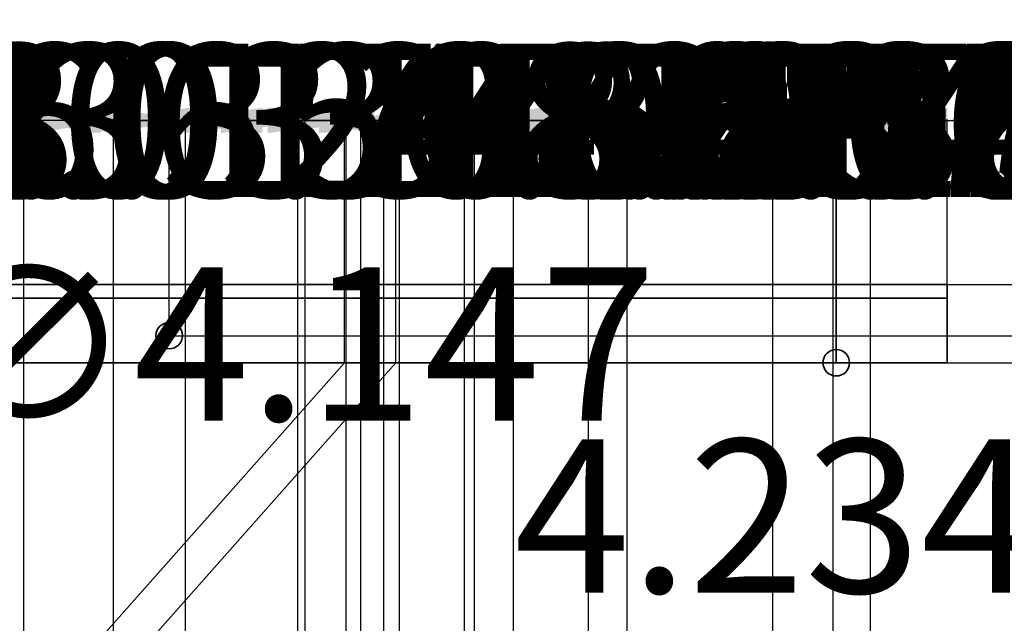
# Model space of a CAD drawing. Units: inches. Extents: x 172 to 828, y 190 to 777.
# Tile 7 of 9: x 474 to 628, y 682 to 777. Entities that reach past the tile are written whole.
import ezdxf

# ---------------------------------------------------------------- set-up
doc = ezdxf.new("R2010")
doc.units = ezdxf.units.IN
doc.header["$MEASUREMENT"] = 0
doc.layers.add('A-ANNO-DIMS', color=2, linetype='Continuous', lineweight=18)
doc.layers.add('A-ELEV', color=7, linetype='Continuous', lineweight=35)
doc.styles.get("Standard").update_dxf_attribs({"font": 'arial.ttf'})
doc.dimstyles.get("Standard").update_dxf_attribs({"dimtxt": 24, "dimasz": 12, "dimexe": 0.18, "dimexo": 0.0625, "dimgap": 0.09, "dimtad": 0, "dimtih": 1, "dimtoh": 1, "dimdec": 0, "dimzin": 0, "dimdsep": 46, "dimlunit": 3, "dimtxsty": 'Standard', "dimcen": 0.09, "dimadec": 0, "dimazin": 0, "dimtfac": 1, "dimtdec": 0, "dimtofl": 0, "dimtmove": 0, "dimatfit": 3, "dimfxl": 1, "dimtolj": 1, "dimtzin": 0, "dimarcsym": 0})

# ---------------------------------------------------------------- blocks, each defined once
blk = doc.blocks.new('*D10')
at = {"layer": 'A-ANNO-DIMS', "color": 0, "lineweight": -2, "transparency": 16777216}
for p, q in [((258.78, 231.45), (258.78, 761.27)), ((270.78, 761.09), (412.23, 761.09)), ((606.78, 761.09), (465.33, 761.09)), ((618.78, 735.45), (618.78, 761.27))]:
    blk.add_line(p, q, dxfattribs=at)
at = {"layer": 'A-ANNO-DIMS', "color": 0, "transparency": 16777216}
for points in [[(270.78, 763.09), (270.78, 759.09), (258.78, 761.09)], [(606.78, 763.09), (606.78, 759.09), (618.78, 761.09)]]:
    blk.add_solid(points, dxfattribs=at)
at = {"layer": 'Defpoints', "color": 0, "transparency": 16777216}
for p in [(618.78, 761.09), (618.78, 735.39), (258.78, 231.39)]:
    blk.add_point(p, dxfattribs=at)
at = {"layer": 'A-ANNO-DIMS', "color": 0, "transparency": 16777216, "insert": (438.78, 761.09), "char_height": 24, "attachment_point": 5}
blk.add_mtext('\\A1;360', dxfattribs=at)
blk = doc.blocks.new('*D11')
at = {"layer": 'A-ANNO-DIMS', "color": 0, "lineweight": -2, "transparency": 16777216}
for p, q in [((618.84, 735.39), (645.16, 735.39)), ((644.98, 723.39), (644.98, 495.74)), ((644.98, 243.39), (644.98, 471.05)), ((618.84, 231.39), (645.16, 231.39))]:
    blk.add_line(p, q, dxfattribs=at)
at = {"layer": 'A-ANNO-DIMS', "color": 0, "transparency": 16777216}
for points in [[(642.98, 723.39), (646.98, 723.39), (644.98, 735.39)], [(642.98, 243.39), (646.98, 243.39), (644.98, 231.39)]]:
    blk.add_solid(points, dxfattribs=at)
at = {"layer": 'Defpoints', "color": 0, "transparency": 16777216}
for p in [(618.78, 735.39), (644.98, 735.39), (618.78, 231.39)]:
    blk.add_point(p, dxfattribs=at)
at = {"layer": 'A-ANNO-DIMS', "color": 0, "transparency": 16777216, "insert": (644.98, 483.39), "char_height": 24, "attachment_point": 5}
blk.add_mtext('\\A1;504', dxfattribs=at)
blk = doc.blocks.new('*D36')
at = {"layer": 'A-ANNO-DIMS', "color": 0, "lineweight": -2, "transparency": 16777216}
for p, q in [((258.78, 735.45), (258.78, 761.27)), ((270.78, 761.09), (412.23, 761.09)), ((606.78, 761.09), (465.33, 761.09)), ((618.78, 735.45), (618.78, 761.27))]:
    blk.add_line(p, q, dxfattribs=at)
at = {"layer": 'A-ANNO-DIMS', "color": 0, "transparency": 16777216}
for points in [[(270.78, 763.09), (270.78, 759.09), (258.78, 761.09)], [(606.78, 763.09), (606.78, 759.09), (618.78, 761.09)]]:
    blk.add_solid(points, dxfattribs=at)
at = {"layer": 'Defpoints', "color": 0, "transparency": 16777216}
for p in [(618.78, 761.09), (258.78, 735.39), (618.78, 735.39)]:
    blk.add_point(p, dxfattribs=at)
at = {"layer": 'A-ANNO-DIMS', "color": 0, "transparency": 16777216, "insert": (438.78, 761.09), "char_height": 24, "attachment_point": 5}
blk.add_mtext('\\A1;360', dxfattribs=at)
blk = doc.blocks.new('*D44')
at = {"layer": 'A-ANNO-DIMS', "color": 0, "lineweight": -2, "transparency": 16777216}
for p, q in [((333.72, 723.23), (333.72, 761.27)), ((345.72, 761.09), (377.1, 761.09)), ((389.1, 727.47), (389.1, 761.27)), ((389.1, 761.09), (401.1, 761.09))]:
    blk.add_line(p, q, dxfattribs=at)
at = {"layer": 'A-ANNO-DIMS', "color": 0, "transparency": 16777216}
for points in [[(345.72, 763.09), (345.72, 759.09), (333.72, 761.09)], [(377.1, 763.09), (377.1, 759.09), (389.1, 761.09)]]:
    blk.add_solid(points, dxfattribs=at)
at = {"layer": 'Defpoints', "color": 0, "transparency": 16777216}
for p in [(389.1, 761.09), (389.1, 727.4), (333.72, 723.17)]:
    blk.add_point(p, dxfattribs=at)
at = {"layer": 'A-ANNO-DIMS', "color": 0, "transparency": 16777216, "insert": (441.71, 761.09), "char_height": 24, "attachment_point": 5}
blk.add_mtext('\\A1;55.38', dxfattribs=at)
blk = doc.blocks.new('*D45')
at = {"layer": 'A-ANNO-DIMS', "color": 0, "lineweight": -2, "transparency": 16777216}
for p, q in [((389.1, 727.47), (389.1, 761.27)), ((401.1, 761.09), (417.14, 761.09)), ((429.14, 615.45), (429.14, 761.27)), ((429.14, 761.09), (441.14, 761.09))]:
    blk.add_line(p, q, dxfattribs=at)
at = {"layer": 'A-ANNO-DIMS', "color": 0, "transparency": 16777216}
for points in [[(401.1, 763.09), (401.1, 759.09), (389.1, 761.09)], [(417.14, 763.09), (417.14, 759.09), (429.14, 761.09)]]:
    blk.add_solid(points, dxfattribs=at)
at = {"layer": 'Defpoints', "color": 0, "transparency": 16777216}
for p in [(429.14, 761.09), (389.1, 727.4), (429.14, 615.39)]:
    blk.add_point(p, dxfattribs=at)
at = {"layer": 'A-ANNO-DIMS', "color": 0, "transparency": 16777216, "insert": (482.2, 761.09), "char_height": 24, "attachment_point": 5}
blk.add_mtext('\\A1;40.03', dxfattribs=at)
blk = doc.blocks.new('*D46')
at = {"layer": 'A-ANNO-DIMS', "color": 0, "lineweight": -2, "transparency": 16777216}
for p, q in [((429.14, 615.45), (429.14, 761.27)), ((441.14, 761.09), (445.77, 761.09)), ((485.14, 761.09), (480.51, 761.09)), ((497.14, 727.47), (497.14, 761.27))]:
    blk.add_line(p, q, dxfattribs=at)
at = {"layer": 'A-ANNO-DIMS', "color": 0, "transparency": 16777216}
for points in [[(441.14, 763.09), (441.14, 759.09), (429.14, 761.09)], [(485.14, 763.09), (485.14, 759.09), (497.14, 761.09)]]:
    blk.add_solid(points, dxfattribs=at)
at = {"layer": 'Defpoints', "color": 0, "transparency": 16777216}
for p in [(497.14, 761.09), (497.14, 727.4), (429.14, 615.39)]:
    blk.add_point(p, dxfattribs=at)
at = {"layer": 'A-ANNO-DIMS', "color": 0, "transparency": 16777216, "insert": (463.14, 761.09), "char_height": 24, "attachment_point": 5}
blk.add_mtext('\\A1;68', dxfattribs=at)
blk = doc.blocks.new('*D47')
at = {"layer": 'A-ANNO-DIMS', "color": 0, "lineweight": -2, "transparency": 16777216}
for p, q in [((497.14, 727.47), (497.14, 761.27)), ((509.14, 761.09), (512.55, 761.09)), ((524.55, 723.23), (524.55, 761.27)), ((524.55, 761.09), (536.55, 761.09))]:
    blk.add_line(p, q, dxfattribs=at)
at = {"layer": 'A-ANNO-DIMS', "color": 0, "transparency": 16777216}
for points in [[(509.14, 763.09), (509.14, 759.09), (497.14, 761.09)], [(512.55, 763.09), (512.55, 759.09), (524.55, 761.09)]]:
    blk.add_solid(points, dxfattribs=at)
at = {"layer": 'Defpoints', "color": 0, "transparency": 16777216}
for p in [(524.55, 761.09), (497.14, 727.4), (524.55, 723.17)]:
    blk.add_point(p, dxfattribs=at)
at = {"layer": 'A-ANNO-DIMS', "color": 0, "transparency": 16777216, "insert": (575.02, 761.09), "char_height": 24, "attachment_point": 5}
blk.add_mtext('\\A1;27.41', dxfattribs=at)
blk = doc.blocks.new('*D48')
at = {"layer": 'A-ANNO-DIMS', "color": 0, "lineweight": -2, "transparency": 16777216}
for p, q in [((512.55, 761.09), (500.55, 761.09)), ((524.55, 723.23), (524.55, 761.27)), ((532.56, 723.23), (532.56, 761.27)), ((544.56, 761.09), (556.56, 761.09))]:
    blk.add_line(p, q, dxfattribs=at)
at = {"layer": 'A-ANNO-DIMS', "color": 0, "transparency": 16777216}
for points in [[(512.55, 763.09), (512.55, 759.09), (524.55, 761.09)], [(544.56, 763.09), (544.56, 759.09), (532.56, 761.09)]]:
    blk.add_solid(points, dxfattribs=at)
at = {"layer": 'Defpoints', "color": 0, "transparency": 16777216}
for p in [(532.56, 761.09), (524.55, 723.17), (532.56, 723.17)]:
    blk.add_point(p, dxfattribs=at)
at = {"layer": 'A-ANNO-DIMS', "color": 0, "transparency": 16777216, "insert": (597.16, 761.09), "char_height": 24, "attachment_point": 5}
blk.add_mtext('\\A1;8.013', dxfattribs=at)
blk = doc.blocks.new('*D49')
at = {"layer": 'A-ANNO-DIMS', "color": 0, "lineweight": -2, "transparency": 16777216}
for p, q in [((520.563677, 761.092291), (508.563677, 761.092291)), ((532.563677, 723.230871), (532.563677, 761.272291)), ((601.465061, 723.230871), (601.465061, 761.272291)), ((613.465061, 761.092291), (625.465061, 761.092291))]:
    blk.add_line(p, q, dxfattribs=at)
at = {"layer": 'A-ANNO-DIMS', "color": 0, "transparency": 16777216}
for points in [[(520.563677, 763.092291), (520.563677, 759.092291), (532.563677, 761.092291)], [(613.465061, 763.092291), (613.465061, 759.092291), (601.465061, 761.092291)]]:
    blk.add_solid(points, dxfattribs=at)
at = {"layer": 'Defpoints', "color": 0, "transparency": 16777216}
for p in [(601.465061, 761.092291), (532.563677, 723.168371), (601.465061, 723.168371)]:
    blk.add_point(p, dxfattribs=at)
at = {"layer": 'A-ANNO-DIMS', "color": 0, "transparency": 16777216, "insert": (567.014369, 761.092291), "char_height": 24, "attachment_point": 5}
blk.add_mtext('\\A1;68.9', dxfattribs=at)
blk = doc.blocks.new('*D50')
at = {"layer": 'A-ANNO-DIMS', "color": 0, "lineweight": -2, "transparency": 16777216}
for p, q in [((589.47, 761.09), (577.47, 761.09)), ((601.47, 723.23), (601.47, 761.27)), ((618.78, 735.45), (618.78, 761.27)), ((630.78, 761.09), (642.78, 761.09))]:
    blk.add_line(p, q, dxfattribs=at)
at = {"layer": 'A-ANNO-DIMS', "color": 0, "transparency": 16777216}
for points in [[(589.47, 763.09), (589.47, 759.09), (601.47, 761.09)], [(630.78, 763.09), (630.78, 759.09), (618.78, 761.09)]]:
    blk.add_solid(points, dxfattribs=at)
at = {"layer": 'Defpoints', "color": 0, "transparency": 16777216}
for p in [(618.78, 761.09), (618.78, 735.39), (601.47, 723.17)]:
    blk.add_point(p, dxfattribs=at)
at = {"layer": 'A-ANNO-DIMS', "color": 0, "transparency": 16777216, "insert": (691.51, 761.09), "char_height": 24, "attachment_point": 5}
blk.add_mtext('\\A1;17.314', dxfattribs=at)
blk = doc.blocks.new('*D51')
at = {"layer": 'A-ANNO-DIMS', "color": 0, "lineweight": -2, "transparency": 16777216}
for p, q in [((644.98, 739.4), (644.98, 751.4)), ((497.2, 727.4), (645.16, 727.4)), ((601.53, 723.17), (645.16, 723.17)), ((644.98, 711.17), (644.98, 699.17)), ((644.98, 699.17), (632.98, 699.17))]:
    blk.add_line(p, q, dxfattribs=at)
at = {"layer": 'A-ANNO-DIMS', "color": 0, "transparency": 16777216}
for points in [[(642.98, 739.4), (646.98, 739.4), (644.98, 727.4)], [(642.98, 711.17), (646.98, 711.17), (644.98, 723.17)]]:
    blk.add_solid(points, dxfattribs=at)
at = {"layer": 'Defpoints', "color": 0, "transparency": 16777216}
for p in [(497.14, 727.4), (601.47, 723.17), (644.98, 723.17)]:
    blk.add_point(p, dxfattribs=at)
at = {"layer": 'A-ANNO-DIMS', "color": 0, "transparency": 16777216, "insert": (591.96, 699.17), "char_height": 24, "attachment_point": 5}
blk.add_mtext('\\A1;4.234', dxfattribs=at)
blk = doc.blocks.new('*D52')
at = {"layer": 'A-ANNO-DIMS', "color": 0, "lineweight": -2, "transparency": 16777216}
for p, q in [((409.12, 761.09), (397.12, 761.09)), ((421.12, 615.45), (421.12, 761.27)), ((429.14, 615.45), (429.14, 761.27)), ((441.14, 761.09), (453.14, 761.09))]:
    blk.add_line(p, q, dxfattribs=at)
at = {"layer": 'A-ANNO-DIMS', "color": 0, "transparency": 16777216}
for points in [[(409.12, 763.09), (409.12, 759.09), (421.12, 761.09)], [(441.14, 763.09), (441.14, 759.09), (429.14, 761.09)]]:
    blk.add_solid(points, dxfattribs=at)
at = {"layer": 'Defpoints', "color": 0, "transparency": 16777216}
for p in [(429.14, 761.09), (421.12, 615.39), (429.14, 615.39)]:
    blk.add_point(p, dxfattribs=at)
at = {"layer": 'A-ANNO-DIMS', "color": 0, "transparency": 16777216, "insert": (493.74, 761.09), "char_height": 24, "attachment_point": 5}
blk.add_mtext('\\A1;8.013', dxfattribs=at)
blk = doc.blocks.new('*D53')
at = {"layer": 'A-ANNO-DIMS', "color": 0, "lineweight": -2, "transparency": 16777216}
for p, q in [((417.14, 761.09), (405.14, 761.09)), ((429.14, 615.45), (429.14, 761.27)), ((437.15, 615.45), (437.15, 761.27)), ((449.15, 761.09), (461.15, 761.09))]:
    blk.add_line(p, q, dxfattribs=at)
at = {"layer": 'A-ANNO-DIMS', "color": 0, "transparency": 16777216}
for points in [[(417.14, 763.09), (417.14, 759.09), (429.14, 761.09)], [(449.15, 763.09), (449.15, 759.09), (437.15, 761.09)]]:
    blk.add_solid(points, dxfattribs=at)
at = {"layer": 'Defpoints', "color": 0, "transparency": 16777216}
for p in [(437.15, 761.09), (429.14, 615.39), (437.15, 615.39)]:
    blk.add_point(p, dxfattribs=at)
at = {"layer": 'A-ANNO-DIMS', "color": 0, "transparency": 16777216, "insert": (501.75, 761.09), "char_height": 24, "attachment_point": 5}
blk.add_mtext('\\A1;8.013', dxfattribs=at)
blk = doc.blocks.new('*D54')
at = {"layer": 'A-ANNO-DIMS', "color": 0, "lineweight": -2, "transparency": 16777216}
for p, q in [((267.48, 615.45), (267.48, 761.27)), ((279.48, 761.09), (330.13, 761.09)), ((462.39, 761.09), (411.75, 761.09)), ((474.39, 633.61), (474.39, 761.27))]:
    blk.add_line(p, q, dxfattribs=at)
at = {"layer": 'A-ANNO-DIMS', "color": 0, "transparency": 16777216}
for points in [[(279.48, 763.09), (279.48, 759.09), (267.48, 761.09)], [(462.39, 763.09), (462.39, 759.09), (474.39, 761.09)]]:
    blk.add_solid(points, dxfattribs=at)
at = {"layer": 'Defpoints', "color": 0, "transparency": 16777216}
for p in [(474.39, 761.09), (474.39, 633.55), (267.48, 615.39)]:
    blk.add_point(p, dxfattribs=at)
at = {"layer": 'A-ANNO-DIMS', "color": 0, "transparency": 16777216, "insert": (370.94, 761.09), "char_height": 24, "attachment_point": 5}
blk.add_mtext('\\A1;206.9', dxfattribs=at)
blk = doc.blocks.new('*D55')
at = {"layer": 'A-ANNO-DIMS', "color": 0, "lineweight": -2, "transparency": 16777216}
for p, q in [((474.39, 633.61), (474.39, 761.27)), ((486.39, 761.09), (506.4, 761.09)), ((518.4, 633.61), (518.4, 761.27)), ((518.4, 761.09), (530.4, 761.09))]:
    blk.add_line(p, q, dxfattribs=at)
at = {"layer": 'A-ANNO-DIMS', "color": 0, "transparency": 16777216}
for points in [[(486.39, 763.09), (486.39, 759.09), (474.39, 761.09)], [(506.4, 763.09), (506.4, 759.09), (518.4, 761.09)]]:
    blk.add_solid(points, dxfattribs=at)
at = {"layer": 'Defpoints', "color": 0, "transparency": 16777216}
for p in [(518.4, 761.09), (474.39, 633.55), (518.4, 633.55)]:
    blk.add_point(p, dxfattribs=at)
at = {"layer": 'A-ANNO-DIMS', "color": 0, "transparency": 16777216, "insert": (569.15, 761.09), "char_height": 24, "attachment_point": 5}
blk.add_mtext('\\A1;44.01', dxfattribs=at)
blk = doc.blocks.new('*D56')
at = {"layer": 'A-ANNO-DIMS', "color": 0, "lineweight": -2, "transparency": 16777216}
for p, q in [((506.4, 761.09), (494.4, 761.09)), ((518.4, 633.61), (518.4, 761.27)), ((527.09, 657.43), (527.09, 761.27)), ((539.09, 761.09), (551.09, 761.09))]:
    blk.add_line(p, q, dxfattribs=at)
at = {"layer": 'A-ANNO-DIMS', "color": 0, "transparency": 16777216}
for points in [[(506.4, 763.09), (506.4, 759.09), (518.4, 761.09)], [(539.09, 763.09), (539.09, 759.09), (527.09, 761.09)]]:
    blk.add_solid(points, dxfattribs=at)
at = {"layer": 'Defpoints', "color": 0, "transparency": 16777216}
for p in [(527.09, 761.09), (527.09, 657.37), (518.4, 633.55)]:
    blk.add_point(p, dxfattribs=at)
at = {"layer": 'A-ANNO-DIMS', "color": 0, "transparency": 16777216, "insert": (582.4, 761.09), "char_height": 24, "attachment_point": 5}
blk.add_mtext('\\A1;8.69', dxfattribs=at)
blk = doc.blocks.new('*D57')
at = {"layer": 'A-ANNO-DIMS', "color": 0, "lineweight": -2, "transparency": 16777216}
for p, q in [((515.09, 761.09), (503.09, 761.09)), ((527.09, 657.43), (527.09, 761.27)), ((533.17, 657.43), (533.17, 761.27)), ((545.17, 761.09), (557.17, 761.09))]:
    blk.add_line(p, q, dxfattribs=at)
at = {"layer": 'A-ANNO-DIMS', "color": 0, "transparency": 16777216}
for points in [[(515.09, 763.09), (515.09, 759.09), (527.09, 761.09)], [(545.17, 763.09), (545.17, 759.09), (533.17, 761.09)]]:
    blk.add_solid(points, dxfattribs=at)
at = {"layer": 'Defpoints', "color": 0, "transparency": 16777216}
for p in [(533.17, 761.09), (527.09, 657.37), (533.17, 657.37)]:
    blk.add_point(p, dxfattribs=at)
at = {"layer": 'A-ANNO-DIMS', "color": 0, "transparency": 16777216, "insert": (597.85, 761.09), "char_height": 24, "attachment_point": 5}
blk.add_mtext('\\A1;6.078', dxfattribs=at)
blk = doc.blocks.new('*D58')
at = {"layer": 'A-ANNO-DIMS', "color": 0, "lineweight": -2, "transparency": 16777216}
for p, q in [((521.17, 761.09), (509.17, 761.09)), ((533.17, 657.43), (533.17, 761.27)), ((544.89, 657.43), (544.89, 761.27)), ((556.89, 761.09), (568.89, 761.09))]:
    blk.add_line(p, q, dxfattribs=at)
at = {"layer": 'A-ANNO-DIMS', "color": 0, "transparency": 16777216}
for points in [[(521.17, 763.09), (521.17, 759.09), (533.17, 761.09)], [(556.89, 763.09), (556.89, 759.09), (544.89, 761.09)]]:
    blk.add_solid(points, dxfattribs=at)
at = {"layer": 'Defpoints', "color": 0, "transparency": 16777216}
for p in [(544.89, 761.09), (533.17, 657.37), (544.89, 657.37)]:
    blk.add_point(p, dxfattribs=at)
at = {"layer": 'A-ANNO-DIMS', "color": 0, "transparency": 16777216, "insert": (608.22, 761.09), "char_height": 24, "attachment_point": 5}
blk.add_mtext('\\A1;11.72', dxfattribs=at)
blk = doc.blocks.new('*D59')
at = {"layer": 'A-ANNO-DIMS', "color": 0, "lineweight": -2, "transparency": 16777216}
for p, q in [((532.89, 761.09), (520.89, 761.09)), ((544.89, 657.43), (544.89, 761.27)), ((550.97, 657.43), (550.97, 761.27)), ((562.97, 761.09), (574.97, 761.09))]:
    blk.add_line(p, q, dxfattribs=at)
at = {"layer": 'A-ANNO-DIMS', "color": 0, "transparency": 16777216}
for points in [[(532.89, 763.09), (532.89, 759.09), (544.89, 761.09)], [(562.97, 763.09), (562.97, 759.09), (550.97, 761.09)]]:
    blk.add_solid(points, dxfattribs=at)
at = {"layer": 'Defpoints', "color": 0, "transparency": 16777216}
for p in [(550.97, 761.09), (544.89, 657.37), (550.97, 657.37)]:
    blk.add_point(p, dxfattribs=at)
at = {"layer": 'A-ANNO-DIMS', "color": 0, "transparency": 16777216, "insert": (615.64, 761.09), "char_height": 24, "attachment_point": 5}
blk.add_mtext('\\A1;6.078', dxfattribs=at)
blk = doc.blocks.new('*D60')
at = {"layer": 'A-ANNO-DIMS', "color": 0, "lineweight": -2, "transparency": 16777216}
for p, q in [((538.97, 761.09), (526.97, 761.09)), ((550.97, 657.43), (550.97, 761.27)), ((562.69, 657.43), (562.69, 761.27)), ((574.69, 761.09), (586.69, 761.09))]:
    blk.add_line(p, q, dxfattribs=at)
at = {"layer": 'A-ANNO-DIMS', "color": 0, "transparency": 16777216}
for points in [[(538.97, 763.09), (538.97, 759.09), (550.97, 761.09)], [(574.69, 763.09), (574.69, 759.09), (562.69, 761.09)]]:
    blk.add_solid(points, dxfattribs=at)
at = {"layer": 'Defpoints', "color": 0, "transparency": 16777216}
for p in [(562.69, 761.09), (550.97, 657.37), (562.69, 657.37)]:
    blk.add_point(p, dxfattribs=at)
at = {"layer": 'A-ANNO-DIMS', "color": 0, "transparency": 16777216, "insert": (626.02, 761.09), "char_height": 24, "attachment_point": 5}
blk.add_mtext('\\A1;11.72', dxfattribs=at)
blk = doc.blocks.new('*D61')
at = {"layer": 'A-ANNO-DIMS', "color": 0, "lineweight": -2, "transparency": 16777216}
for p, q in [((550.69, 761.09), (538.69, 761.09)), ((562.69, 657.43), (562.69, 761.27)), ((568.77, 657.43), (568.77, 761.27)), ((580.77, 761.09), (592.77, 761.09))]:
    blk.add_line(p, q, dxfattribs=at)
at = {"layer": 'A-ANNO-DIMS', "color": 0, "transparency": 16777216}
for points in [[(550.69, 763.09), (550.69, 759.09), (562.69, 761.09)], [(580.77, 763.09), (580.77, 759.09), (568.77, 761.09)]]:
    blk.add_solid(points, dxfattribs=at)
at = {"layer": 'Defpoints', "color": 0, "transparency": 16777216}
for p in [(568.77, 761.09), (562.69, 657.37), (568.77, 657.37)]:
    blk.add_point(p, dxfattribs=at)
at = {"layer": 'A-ANNO-DIMS', "color": 0, "transparency": 16777216, "insert": (633.44, 761.09), "char_height": 24, "attachment_point": 5}
blk.add_mtext('\\A1;6.078', dxfattribs=at)
blk = doc.blocks.new('*D62')
at = {"layer": 'A-ANNO-DIMS', "color": 0, "lineweight": -2, "transparency": 16777216}
for p, q in [((568.77, 657.43), (568.77, 761.27)), ((580.77, 761.09), (594.82, 761.09)), ((606.82, 663.45), (606.82, 761.27)), ((606.82, 761.09), (618.82, 761.09))]:
    blk.add_line(p, q, dxfattribs=at)
at = {"layer": 'A-ANNO-DIMS', "color": 0, "transparency": 16777216}
for points in [[(580.77, 763.09), (580.77, 759.09), (568.77, 761.09)], [(594.82, 763.09), (594.82, 759.09), (606.82, 761.09)]]:
    blk.add_solid(points, dxfattribs=at)
at = {"layer": 'Defpoints', "color": 0, "transparency": 16777216}
for p in [(606.82, 761.09), (606.82, 663.39), (568.77, 657.37)]:
    blk.add_point(p, dxfattribs=at)
at = {"layer": 'A-ANNO-DIMS', "color": 0, "transparency": 16777216, "insert": (659.48, 761.09), "char_height": 24, "attachment_point": 5}
blk.add_mtext('\\A1;38.05', dxfattribs=at)
blk = doc.blocks.new('*D63')
at = {"layer": 'A-ANNO-DIMS', "color": 0, "lineweight": -2, "transparency": 16777216}
for p, q in [((594.82, 761.09), (582.82, 761.09)), ((606.82, 663.45), (606.82, 761.27)), ((618.78, 723.23), (618.78, 761.27)), ((630.78, 761.09), (642.78, 761.09))]:
    blk.add_line(p, q, dxfattribs=at)
at = {"layer": 'A-ANNO-DIMS', "color": 0, "transparency": 16777216}
for points in [[(594.82, 763.09), (594.82, 759.09), (606.82, 761.09)], [(630.78, 763.09), (630.78, 759.09), (618.78, 761.09)]]:
    blk.add_solid(points, dxfattribs=at)
at = {"layer": 'Defpoints', "color": 0, "transparency": 16777216}
for p in [(618.78, 761.09), (618.78, 723.17), (606.82, 663.39)]:
    blk.add_point(p, dxfattribs=at)
at = {"layer": 'A-ANNO-DIMS', "color": 0, "transparency": 16777216, "insert": (691.56, 761.09), "char_height": 24, "attachment_point": 5}
blk.add_mtext('\\A1;11.963', dxfattribs=at)
blk = doc.blocks.new('*D76')
at = {"layer": 'A-ANNO-DIMS', "color": 0, "lineweight": -2, "transparency": 16777216}
for p, q in [((399.24, 761.09), (387.24, 761.09)), ((411.24, 495.45), (411.24, 761.27)), ((427.59, 495.45), (427.59, 761.27)), ((439.59, 761.09), (451.59, 761.09))]:
    blk.add_line(p, q, dxfattribs=at)
at = {"layer": 'A-ANNO-DIMS', "color": 0, "transparency": 16777216}
for points in [[(399.24, 763.09), (399.24, 759.09), (411.24, 761.09)], [(439.59, 763.09), (439.59, 759.09), (427.59, 761.09)]]:
    blk.add_solid(points, dxfattribs=at)
at = {"layer": 'Defpoints', "color": 0, "transparency": 16777216}
for p in [(427.59, 761.09), (411.24, 495.39), (427.59, 495.39)]:
    blk.add_point(p, dxfattribs=at)
at = {"layer": 'A-ANNO-DIMS', "color": 0, "transparency": 16777216, "insert": (500.36, 761.09), "char_height": 24, "attachment_point": 5}
blk.add_mtext('\\A1;16.356', dxfattribs=at)
blk = doc.blocks.new('*D77')
at = {"layer": 'A-ANNO-DIMS', "color": 0, "lineweight": -2, "transparency": 16777216}
for p, q in [((427.59, 495.45), (427.59, 761.27)), ((439.59, 761.09), (452.34, 761.09)), ((464.34, 495.45), (464.34, 761.27)), ((464.34, 761.09), (476.34, 761.09))]:
    blk.add_line(p, q, dxfattribs=at)
at = {"layer": 'A-ANNO-DIMS', "color": 0, "transparency": 16777216}
for points in [[(439.59, 763.09), (439.59, 759.09), (427.59, 761.09)], [(452.34, 763.09), (452.34, 759.09), (464.34, 761.09)]]:
    blk.add_solid(points, dxfattribs=at)
at = {"layer": 'Defpoints', "color": 0, "transparency": 16777216}
for p in [(464.34, 761.09), (427.59, 495.39), (464.34, 495.39)]:
    blk.add_point(p, dxfattribs=at)
at = {"layer": 'A-ANNO-DIMS', "color": 0, "transparency": 16777216, "insert": (516.86, 761.09), "char_height": 24, "attachment_point": 5}
blk.add_mtext('\\A1;36.74', dxfattribs=at)
blk = doc.blocks.new('*D78')
at = {"layer": 'A-ANNO-DIMS', "color": 0, "lineweight": -2, "transparency": 16777216}
for p, q in [((452.34, 761.09), (440.34, 761.09)), ((464.34, 607.45), (464.34, 761.27)), ((488.42, 607.45), (488.42, 761.27)), ((500.42, 761.09), (512.42, 761.09))]:
    blk.add_line(p, q, dxfattribs=at)
at = {"layer": 'A-ANNO-DIMS', "color": 0, "transparency": 16777216}
for points in [[(452.34, 763.09), (452.34, 759.09), (464.34, 761.09)], [(500.42, 763.09), (500.42, 759.09), (488.42, 761.09)]]:
    blk.add_solid(points, dxfattribs=at)
at = {"layer": 'Defpoints', "color": 0, "transparency": 16777216}
for p in [(488.42, 761.09), (464.34, 607.39), (488.42, 607.39)]:
    blk.add_point(p, dxfattribs=at)
at = {"layer": 'A-ANNO-DIMS', "color": 0, "transparency": 16777216, "insert": (562.56, 761.09), "char_height": 24, "attachment_point": 5}
blk.add_mtext('\\A1;24.088', dxfattribs=at)
blk = doc.blocks.new('*D79')
at = {"layer": 'A-ANNO-DIMS', "color": 0, "lineweight": -2, "transparency": 16777216}
for p, q in [((476.42, 761.09), (464.42, 761.09)), ((488.42, 607.45), (488.42, 761.27)), ((499.69, 607.45), (499.69, 761.27)), ((511.69, 761.09), (523.69, 761.09))]:
    blk.add_line(p, q, dxfattribs=at)
at = {"layer": 'A-ANNO-DIMS', "color": 0, "transparency": 16777216}
for points in [[(476.42, 763.09), (476.42, 759.09), (488.42, 761.09)], [(511.69, 763.09), (511.69, 759.09), (499.69, 761.09)]]:
    blk.add_solid(points, dxfattribs=at)
at = {"layer": 'Defpoints', "color": 0, "transparency": 16777216}
for p in [(499.69, 761.09), (488.42, 607.39), (499.69, 607.39)]:
    blk.add_point(p, dxfattribs=at)
at = {"layer": 'A-ANNO-DIMS', "color": 0, "transparency": 16777216, "insert": (563.15, 761.09), "char_height": 24, "attachment_point": 5}
blk.add_mtext('\\A1;11.27', dxfattribs=at)
blk = doc.blocks.new('*D80')
at = {"layer": 'A-ANNO-DIMS', "color": 0, "lineweight": -2, "transparency": 16777216}
for p, q in [((487.69, 761.09), (475.69, 761.09)), ((499.69, 607.45), (499.69, 761.27)), ((517.23, 607.45), (517.23, 761.27)), ((529.23, 761.09), (541.23, 761.09))]:
    blk.add_line(p, q, dxfattribs=at)
at = {"layer": 'A-ANNO-DIMS', "color": 0, "transparency": 16777216}
for points in [[(487.69, 763.09), (487.69, 759.09), (499.69, 761.09)], [(529.23, 763.09), (529.23, 759.09), (517.23, 761.09)]]:
    blk.add_solid(points, dxfattribs=at)
at = {"layer": 'Defpoints', "color": 0, "transparency": 16777216}
for p in [(517.23, 761.09), (499.69, 607.39), (517.23, 607.39)]:
    blk.add_point(p, dxfattribs=at)
at = {"layer": 'A-ANNO-DIMS', "color": 0, "transparency": 16777216, "insert": (590, 761.09), "char_height": 24, "attachment_point": 5}
blk.add_mtext('\\A1;17.533', dxfattribs=at)
blk = doc.blocks.new('*D81')
at = {"layer": 'A-ANNO-DIMS', "color": 0, "lineweight": -2, "transparency": 16777216}
for p, q in [((505.23, 761.09), (493.23, 761.09)), ((517.23, 607.45), (517.23, 761.27)), ((524.83, 493.45), (524.83, 761.27)), ((536.83, 761.09), (548.83, 761.09))]:
    blk.add_line(p, q, dxfattribs=at)
at = {"layer": 'A-ANNO-DIMS', "color": 0, "transparency": 16777216}
for points in [[(505.23, 763.09), (505.23, 759.09), (517.23, 761.09)], [(536.83, 763.09), (536.83, 759.09), (524.83, 761.09)]]:
    blk.add_solid(points, dxfattribs=at)
at = {"layer": 'Defpoints', "color": 0, "transparency": 16777216}
for p in [(524.83, 761.09), (517.23, 607.39), (524.83, 493.39)]:
    blk.add_point(p, dxfattribs=at)
at = {"layer": 'A-ANNO-DIMS', "color": 0, "transparency": 16777216, "insert": (570.66, 761.09), "char_height": 24, "attachment_point": 5}
blk.add_mtext('\\A1;7.6', dxfattribs=at)
blk = doc.blocks.new('*D82')
at = {"layer": 'A-ANNO-DIMS', "color": 0, "lineweight": -2, "transparency": 16777216}
for p, q in [((588.96, 761.09), (576.96, 761.09)), ((600.96, 493.45), (600.96, 761.27)), ((606.82, 607.45), (606.82, 761.27)), ((618.82, 761.09), (630.82, 761.09))]:
    blk.add_line(p, q, dxfattribs=at)
at = {"layer": 'A-ANNO-DIMS', "color": 0, "transparency": 16777216}
for points in [[(588.96, 763.09), (588.96, 759.09), (600.96, 761.09)], [(618.82, 763.09), (618.82, 759.09), (606.82, 761.09)]]:
    blk.add_solid(points, dxfattribs=at)
at = {"layer": 'Defpoints', "color": 0, "transparency": 16777216}
for p in [(606.82, 761.09), (606.82, 607.39), (600.96, 493.39)]:
    blk.add_point(p, dxfattribs=at)
at = {"layer": 'A-ANNO-DIMS', "color": 0, "transparency": 16777216, "insert": (671.39, 761.09), "char_height": 24, "attachment_point": 5}
blk.add_mtext('\\A1;5.856', dxfattribs=at)
blk = doc.blocks.new('*D83')
at = {"layer": 'A-ANNO-DIMS', "color": 0, "lineweight": -2, "transparency": 16777216}
for p, q in [((512.83, 761.09), (500.83, 761.09)), ((524.83, 535.45), (524.83, 761.27)), ((543.3, 599.86), (543.3, 761.27)), ((555.3, 761.09), (567.3, 761.09))]:
    blk.add_line(p, q, dxfattribs=at)
at = {"layer": 'A-ANNO-DIMS', "color": 0, "transparency": 16777216}
for points in [[(512.83, 763.09), (512.83, 759.09), (524.83, 761.09)], [(555.3, 763.09), (555.3, 759.09), (543.3, 761.09)]]:
    blk.add_solid(points, dxfattribs=at)
at = {"layer": 'Defpoints', "color": 0, "transparency": 16777216}
for p in [(543.3, 761.09), (543.3, 599.8), (524.83, 535.39)]:
    blk.add_point(p, dxfattribs=at)
at = {"layer": 'A-ANNO-DIMS', "color": 0, "transparency": 16777216, "insert": (606.75, 761.09), "char_height": 24, "attachment_point": 5}
blk.add_mtext('\\A1;18.47', dxfattribs=at)
blk = doc.blocks.new('*D84')
at = {"layer": 'A-ANNO-DIMS', "color": 0, "lineweight": -2, "transparency": 16777216}
for p, q in [((543.3, 599.86), (543.3, 761.27)), ((555.3, 761.09), (579.54, 761.09)), ((591.54, 599.86), (591.54, 761.27)), ((591.54, 761.09), (603.54, 761.09))]:
    blk.add_line(p, q, dxfattribs=at)
at = {"layer": 'A-ANNO-DIMS', "color": 0, "transparency": 16777216}
for points in [[(555.3, 763.09), (555.3, 759.09), (543.3, 761.09)], [(579.54, 763.09), (579.54, 759.09), (591.54, 761.09)]]:
    blk.add_solid(points, dxfattribs=at)
at = {"layer": 'Defpoints', "color": 0, "transparency": 16777216}
for p in [(591.54, 761.09), (543.3, 599.8), (591.54, 599.8)]:
    blk.add_point(p, dxfattribs=at)
at = {"layer": 'A-ANNO-DIMS', "color": 0, "transparency": 16777216, "insert": (644.7, 761.09), "char_height": 24, "attachment_point": 5}
blk.add_mtext('\\A1;48.25', dxfattribs=at)
blk = doc.blocks.new('*D85')
at = {"layer": 'A-ANNO-DIMS', "color": 0, "lineweight": -2, "transparency": 16777216}
for p, q in [((579.54, 761.09), (567.54, 761.09)), ((591.54, 599.86), (591.54, 761.27)), ((600.96, 535.45), (600.96, 761.27)), ((612.96, 761.09), (624.96, 761.09))]:
    blk.add_line(p, q, dxfattribs=at)
at = {"layer": 'A-ANNO-DIMS', "color": 0, "transparency": 16777216}
for points in [[(579.54, 763.09), (579.54, 759.09), (591.54, 761.09)], [(612.96, 763.09), (612.96, 759.09), (600.96, 761.09)]]:
    blk.add_solid(points, dxfattribs=at)
at = {"layer": 'Defpoints', "color": 0, "transparency": 16777216}
for p in [(600.96, 761.09), (591.54, 599.8), (600.96, 535.39)]:
    blk.add_point(p, dxfattribs=at)
at = {"layer": 'A-ANNO-DIMS', "color": 0, "transparency": 16777216, "insert": (665.63, 761.09), "char_height": 24, "attachment_point": 5}
blk.add_mtext('\\A1;9.415', dxfattribs=at)
blk = doc.blocks.new('*D86')
at = {"layer": 'A-ANNO-DIMS', "color": 0, "lineweight": -2, "transparency": 16777216}
for p, q in [((512.83, 761.09), (500.83, 761.09)), ((524.83, 493.45), (524.83, 761.27)), ((530.68, 493.45), (530.68, 761.27)), ((542.68, 761.09), (554.68, 761.09))]:
    blk.add_line(p, q, dxfattribs=at)
at = {"layer": 'A-ANNO-DIMS', "color": 0, "transparency": 16777216}
for points in [[(512.83, 763.09), (512.83, 759.09), (524.83, 761.09)], [(542.68, 763.09), (542.68, 759.09), (530.68, 761.09)]]:
    blk.add_solid(points, dxfattribs=at)
at = {"layer": 'Defpoints', "color": 0, "transparency": 16777216}
for p in [(530.68, 761.09), (524.83, 493.39), (530.68, 493.39)]:
    blk.add_point(p, dxfattribs=at)
at = {"layer": 'A-ANNO-DIMS', "color": 0, "transparency": 16777216, "insert": (595.26, 761.09), "char_height": 24, "attachment_point": 5}
blk.add_mtext('\\A1;5.856', dxfattribs=at)
blk = doc.blocks.new('*D92')
at = {"layer": 'A-ANNO-DIMS', "color": 0, "lineweight": -2, "transparency": 16777216}
for p, q in [((389.01, 727.4), (389.19, 727.4)), ((389.1, 727.31), (389.1, 727.49)), ((415.15, 726.11), (403.16, 726.7))]:
    blk.add_line(p, q, dxfattribs=at)
at = {"layer": 'A-ANNO-DIMS', "color": 0, "transparency": 16777216}
blk.add_solid([(403.26, 728.7), (403.06, 724.71), (391.17, 727.3)], dxfattribs=at)
at = {"layer": 'Defpoints', "color": 0, "transparency": 16777216}
for p in [(387.03, 727.51), (391.17, 727.3)]:
    blk.add_point(p, dxfattribs=at)
at = {"layer": 'A-ANNO-DIMS', "color": 0, "transparency": 16777216, "insert": (493.92, 726.11), "char_height": 24, "attachment_point": 5}
blk.add_mtext('\\A1;3X ∅4.147', dxfattribs=at)

msp = doc.modelspace()

# ---------------------------------------------------------------- linework, layer by layer
at = {"layer": 'A-ELEV'}
for p, q in [((618.7792, 735.3923), (267.4822, 735.3923)), ((618.7792, 735.3923), (618.7792, 733.2598)), ((618.7792, 733.2598), (258.7792, 733.2598)), ((618.7792, 733.2598), (618.7792, 723.1684)), ((618.7792, 723.1684), (258.7792, 723.1684)), ((429.1355, 615.3923), (524.5502, 723.1684)), ((437.149, 615.3923), (532.5637, 723.1684))]:
    msp.add_line(p, q, dxfattribs=at)
for centre in [(497.1421, 727.4027), (601.4651, 723.1684)]:
    msp.add_circle(centre, 2.0735, dxfattribs=at)

# ---------------------------------------------------------------- dimensions: what is measured, and where the dimension line sits
at = {"layer": 'A-ANNO-DIMS'}
for base, p1, p2, override, picture, middle in [((618.7792, 761.0923), (258.7792, 231.3923), (618.7792, 735.3923), {"dimdec": 0, "dimlfac": 1, "dimrnd": 0, "dimzin": 0, "dimdsep": 46, "dimlunit": 2}, '*D10', (438.7792, 761.0923)), ((618.7792, 761.0923), (258.7792, 735.3923), (618.7792, 735.3923), {"dimdec": 0, "dimlfac": 1, "dimrnd": 0, "dimzin": 0, "dimdsep": 46, "dimlunit": 2}, '*D36', (438.7792, 761.0923)), ((474.3939, 761.0923), (267.4822, 615.3923), (474.3939, 633.5521), {"dimdec": 1, "dimlfac": 1, "dimrnd": 0, "dimzin": 0, "dimdsep": 46, "dimlunit": 2}, '*D54', (370.9381, 761.0923)), ((389.104, 761.0923), (333.7209, 723.1684), (389.104, 727.4027), {"dimdec": 2, "dimlfac": 1, "dimrnd": 0, "dimzin": 0, "dimdsep": 46, "dimlunit": 2}, '*D44', (441.7124, 761.0923)), ((427.5926, 761.0923), (411.2362, 495.3923), (427.5926, 495.3923), {"dimdec": 3, "dimlfac": 1, "dimrnd": 0, "dimzin": 0, "dimdsep": 46, "dimlunit": 2}, '*D76', (500.362, 761.0923)), ((429.1355, 761.0923), (389.104, 727.4027), (429.1355, 615.3923), {"dimdec": 2, "dimlfac": 1, "dimrnd": 0, "dimzin": 0, "dimdsep": 46, "dimlunit": 2}, '*D45', (482.2024, 761.0923)), ((429.1355, 761.0923), (421.1221, 615.3923), (429.1355, 615.3923), {"dimdec": 3, "dimlfac": 1, "dimrnd": 0, "dimzin": 0, "dimdsep": 46, "dimlunit": 2}, '*D52', (493.7358, 761.0923)), ((437.149, 761.09229), (429.13555, 615.39229), (437.149, 615.39229), {"dimdec": 3, "dimlfac": 1, "dimrnd": 0, "dimzin": 0, "dimdsep": 46, "dimlunit": 2}, '*D53', (501.74924, 761.09229)), ((464.3356, 761.0923), (427.5926, 495.3923), (464.3356, 495.3923), {"dimdec": 2, "dimlfac": 1, "dimrnd": 0, "dimzin": 0, "dimdsep": 46, "dimlunit": 2}, '*D77', (516.8622, 761.0923)), ((497.1421, 761.0923), (429.1355, 615.3923), (497.1421, 727.4027), {"dimdec": 0, "dimlfac": 1, "dimrnd": 0, "dimzin": 0, "dimdsep": 46, "dimlunit": 2}, '*D46', (463.1388, 761.0923)), ((488.4232, 761.0923), (464.3356, 607.3923), (488.4232, 607.3923), {"dimdec": 3, "dimlfac": 1, "dimrnd": 0, "dimzin": 0, "dimdsep": 46, "dimlunit": 2}, '*D78', (562.5596, 761.0923)), ((499.6941, 761.0923), (488.4232, 607.3923), (499.6941, 607.3923), {"dimdec": 2, "dimlfac": 1, "dimrnd": 0, "dimzin": 0, "dimdsep": 46, "dimlunit": 2}, '*D79', (563.1484, 761.0923)), ((518.4045, 761.0923), (474.3939, 633.5521), (518.4045, 633.5521), {"dimdec": 2, "dimlfac": 1, "dimrnd": 0, "dimzin": 0, "dimdsep": 46, "dimlunit": 2}, '*D55', (569.1548, 761.0923)), ((517.2267, 761.0923), (499.6941, 607.3923), (517.2267, 607.3923), {"dimdec": 3, "dimlfac": 1, "dimrnd": 0, "dimzin": 0, "dimdsep": 46, "dimlunit": 2}, '*D80', (590.0043, 761.0923)), ((524.8269, 761.0923), (517.2267, 607.3923), (524.8269, 493.3923), {"dimdec": 1, "dimlfac": 1, "dimrnd": 0, "dimzin": 0, "dimdsep": 46, "dimlunit": 2}, '*D81', (570.6577, 761.0923)), ((527.0943, 761.0923), (518.4045, 633.5521), (527.0943, 657.3703), {"dimdec": 2, "dimlfac": 1, "dimrnd": 0, "dimzin": 0, "dimdsep": 46, "dimlunit": 2}, '*D56', (582.3957, 761.0923)), ((524.5502, 761.0923), (497.1421, 727.4027), (524.5502, 723.1684), {"dimdec": 2, "dimlfac": 1, "dimrnd": 0, "dimzin": 0, "dimdsep": 46, "dimlunit": 2}, '*D47', (575.0222, 761.0923)), ((532.56368, 761.09229), (524.55022, 723.16837), (532.56368, 723.16837), {"dimdec": 3, "dimlfac": 1, "dimrnd": 0, "dimzin": 0, "dimdsep": 46, "dimlunit": 2}, '*D48', (597.16391, 761.09229)), ((543.2956, 761.0923), (524.8269, 535.3923), (543.2956, 599.8013), {"dimdec": 2, "dimlfac": 1, "dimrnd": 0, "dimzin": 0, "dimdsep": 46, "dimlunit": 2}, '*D83', (606.7498, 761.0923)), ((530.6832, 761.0923), (524.8269, 493.3923), (530.6832, 493.3923), {"dimdec": 3, "dimlfac": 1, "dimrnd": 0, "dimzin": 0, "dimdsep": 46, "dimlunit": 2}, '*D86', (595.2589, 761.0923)), ((533.1719, 761.0923), (527.0943, 657.3703), (533.1719, 657.3703), {"dimdec": 3, "dimlfac": 1, "dimrnd": 0, "dimzin": 0, "dimdsep": 46, "dimlunit": 2}, '*D57', (597.8458, 761.0923)), ((601.4651, 761.0923), (532.5637, 723.1684), (601.4651, 723.1684), {"dimdec": 1, "dimlfac": 1, "dimrnd": 0, "dimzin": 0, "dimdsep": 46, "dimlunit": 2}, '*D49', (567.0144, 761.0923)), ((544.8929, 761.0923), (533.1719, 657.3703), (544.8929, 657.3703), {"dimdec": 2, "dimlfac": 1, "dimrnd": 0, "dimzin": 0, "dimdsep": 46, "dimlunit": 2}, '*D58', (608.2244, 761.0923)), ((550.9705, 761.0923), (544.8929, 657.3703), (550.9705, 657.3703), {"dimdec": 3, "dimlfac": 1, "dimrnd": 0, "dimzin": 0, "dimdsep": 46, "dimlunit": 2}, '*D59', (615.6444, 761.0923)), ((562.6916, 761.0923), (550.9705, 657.3703), (562.6916, 657.3703), {"dimdec": 2, "dimlfac": 1, "dimrnd": 0, "dimzin": 0, "dimdsep": 46, "dimlunit": 2}, '*D60', (626.023, 761.0923)), ((568.7692, 761.0923), (562.6916, 657.3703), (568.7692, 657.3703), {"dimdec": 3, "dimlfac": 1, "dimrnd": 0, "dimzin": 0, "dimdsep": 46, "dimlunit": 2}, '*D61', (633.4431, 761.0923)), ((591.5446, 761.0923), (543.2956, 599.8013), (591.5446, 599.8013), {"dimdec": 2, "dimlfac": 1, "dimrnd": 0, "dimzin": 0, "dimdsep": 46, "dimlunit": 2}, '*D84', (644.7014, 761.0923)), ((600.9594, 761.0923), (591.5446, 599.8013), (600.9594, 535.3923), {"dimdec": 3, "dimlfac": 1, "dimrnd": 0, "dimzin": 0, "dimdsep": 46, "dimlunit": 2}, '*D85', (665.6333, 761.0923)), ((606.8158, 761.0923), (568.7692, 657.3703), (606.8158, 663.3923), {"dimdec": 2, "dimlfac": 1, "dimrnd": 0, "dimzin": 0, "dimdsep": 46, "dimlunit": 2}, '*D62', (659.4815, 761.0923)), ((606.8158, 761.0923), (600.9594, 493.3923), (606.8158, 607.3923), {"dimdec": 3, "dimlfac": 1, "dimrnd": 0, "dimzin": 0, "dimdsep": 46, "dimlunit": 2}, '*D82', (671.3915, 761.0923)), ((618.7792, 761.0923), (601.4651, 723.1684), (618.7792, 735.3923), {"dimdec": 3, "dimlfac": 1, "dimrnd": 0, "dimzin": 0, "dimdsep": 46, "dimlunit": 2}, '*D50', (691.5076, 761.0923)), ((618.7792, 761.0923), (606.8158, 663.3923), (618.7792, 723.1684), {"dimdec": 3, "dimlfac": 1, "dimrnd": 0, "dimzin": 0, "dimdsep": 46, "dimlunit": 2}, '*D63', (691.5568, 761.0923))]:
    dim = msp.add_linear_dim(base=base, p1=p1, p2=p2, dimstyle='Standard', override=override, dxfattribs=at)
    dim.commit()
    dim.dimension.update_dxf_attribs({"geometry": picture, "text_midpoint": middle})
dim = msp.add_diameter_dim_2p(p1=(387.033, 727.5056), p2=(391.1749, 727.2998), text='3X <>', dimstyle='Standard', override={"dimdec": 3, "dimlfac": 1, "dimrnd": 0, "dimzin": 0, "dimdsep": 46, "dimlunit": 2}, dxfattribs=at)
dim.commit()
dim.dimension.update_dxf_attribs({"geometry": '*D92', "text_midpoint": (415.1453, 726.1083), "dimtype": 163})
for base, p1, p2, override, picture, middle in [((644.9792, 723.1684), (497.1421, 727.4027), (601.4651, 723.1684), {"dimdec": 3, "dimlfac": 1, "dimrnd": 0, "dimzin": 0, "dimdsep": 46, "dimlunit": 2}, '*D51', (591.9615, 699.1684)), ((644.9792, 735.3923), (618.7792, 231.3923), (618.7792, 735.3923), {"dimdec": 0, "dimlfac": 1, "dimrnd": 0, "dimzin": 0, "dimdsep": 46, "dimlunit": 2}, '*D11', (644.9792, 483.3923))]:
    dim = msp.add_linear_dim(base=base, p1=p1, p2=p2, angle=90, dimstyle='Standard', override=override, dxfattribs=at)
    dim.commit()
    dim.dimension.update_dxf_attribs({"geometry": picture, "text_midpoint": middle})

doc.saveas('drawing.dxf')
